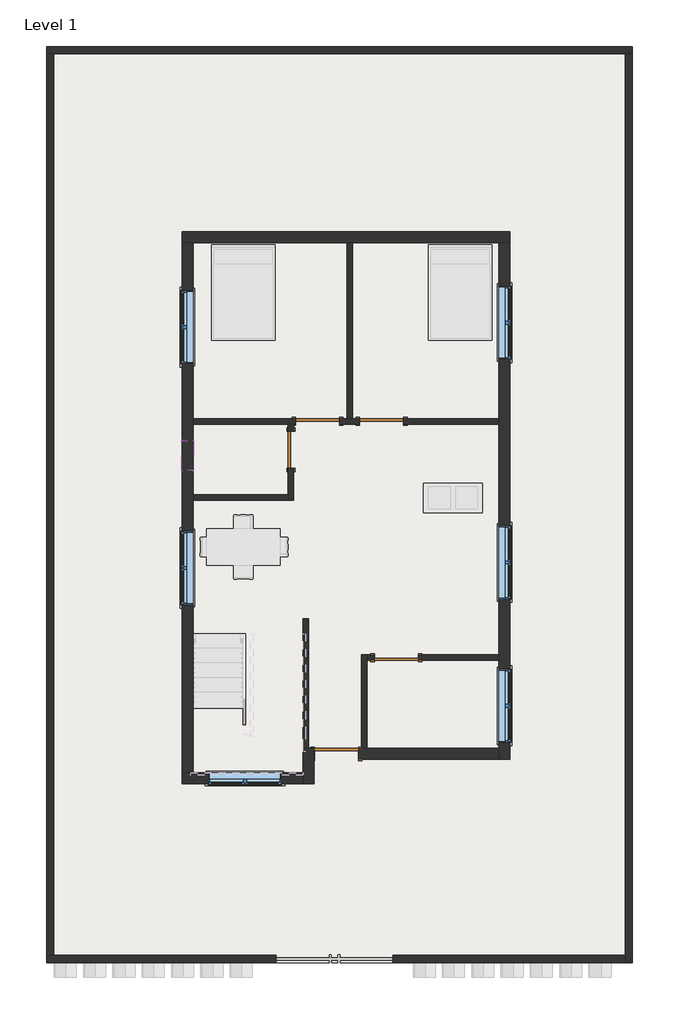
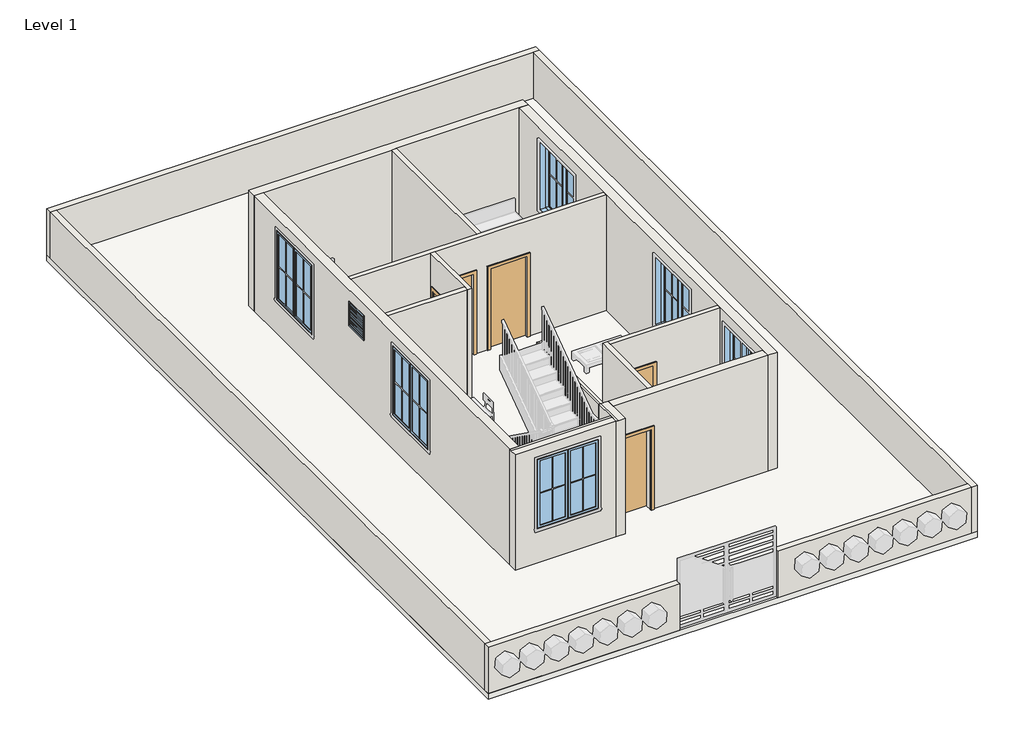
# One storey, part 1 of 3: 18 walls, 7 windows, 5 doors, 1 slab.
"""IFC4 building model written with IfcOpenShell, lengths in millimetres."""

from ifc_helpers import new_model, si_unit, frame, origin, origin_with_axes, place, context, project, spatial, polyline, outline, extrude, faceted_brep, transform, mapped, element, save
from components import door_214872d5, single_flush_door_3_e5f9f3c4, single_flush_door_3_305aa2a5, single_flush_door_3_0ca8825f, window_casement_double_win_5_f93960c7, window_f2d8fef0

model = new_model("IFC4")

# Units and contexts
model_context = context("Model", 3, world=origin())
ifc_project = project(units=[si_unit("LENGTHUNIT", "METRE", prefix="MILLI")], contexts=[model_context])

# Site, building, storey
site = spatial("IfcSite", under=ifc_project)
building = spatial("IfcBuilding", under=site)
storey = spatial("IfcBuildingStorey", under=building, Name="Level 1", Elevation=0.0)

# Doors
placement = place(None, origin())
door_shape = door_214872d5(model_context)
element("IfcDoor", 1, ObjectType="Single-Flush : DOOR 2'6\"", at=placement, inside=storey, context=model_context, shape_type="MappedRepresentation", body=[
    mapped(door_shape, transform((-2193.930864, 251.0919982, 0.0), x_axis=(0.0, 1.0, 0.0), y_axis=(-1.0, 0.0, 0.0), z_axis=(0.0, 0.0, 1.0))),
])
single_flush_door_3_shape = single_flush_door_3_e5f9f3c4(model_context)
element("IfcDoor", 2, ObjectType="Single-Flush : DOOR 3'", at=placement, inside=storey, context=model_context, shape_type="MappedRepresentation", body=[
    mapped(single_flush_door_3_shape, transform((-1641.3962678, 841.6419982, 0.0), x_axis=(1.0, 0.0, 0.0), y_axis=(0.0, 1.0, 0.0), z_axis=(0.0, 0.0, 1.0))),
])
element("IfcDoor", 3, ObjectType="Single-Flush : DOOR 3'", at=placement, inside=storey, context=model_context, shape_type="MappedRepresentation", body=[
    mapped(single_flush_door_3_shape, transform((-3.180864, -4073.2580018, 0.0), x_axis=(-1.0, 0.0, 0.0), y_axis=(0.0, -1.0, 0.0), z_axis=(0.0, 0.0, 1.0))),
])
single_flush_door_3_2_shape = single_flush_door_3_305aa2a5(model_context)
element("IfcDoor", 4, ObjectType="Single-Flush : DOOR 3'", at=placement, inside=storey, context=model_context, shape_type="MappedRepresentation", body=[
    mapped(single_flush_door_3_2_shape, transform((-307.980864, 841.6419982, 0.0), x_axis=(-1.0, 0.0, 0.0), y_axis=(0.0, -1.0, 0.0), z_axis=(0.0, 0.0, 1.0))),
])
single_flush_door_3_3_shape = single_flush_door_3_0ca8825f(model_context)
element("IfcDoor", 5, ObjectType="Single-Flush : DOOR 3'", at=placement, inside=storey, context=model_context, shape_type="MappedRepresentation", body=[
    mapped(single_flush_door_3_3_shape, transform((-1250.955864, -6073.5080018, 0.0), x_axis=(1.0, 0.0, 0.0), y_axis=(0.0, 1.0, 0.0), z_axis=(0.0, 0.0, 1.0))),
])

# Slab
element("IfcSlab", 6, ObjectType="FLOOR 6\"", at=placement, inside=storey, context=model_context, shape_type="SweptSolid", body=[
    extrude(outline(polyline([(4911.0485399, 8634.4627566), (4911.0485399, -10415.5372434), (-7280.9514601, -10415.5372434), (-7280.9514601, 8634.4627566), (4911.0485399, 8634.4627566)])), frame((0.0, 0.0, -152.4), z_axis=(0.0, 0.0, 1.0), x_axis=(1.0, 0.0, 0.0)), (0.0, 0.0, 1.0), 152.4),
])

# Walls
element("IfcWall", 7, ObjectType="CMD 6\"", at=placement, inside=storey, context=model_context, shape_type="Brep", body=[
    faceted_brep([(-7280.9514601, 8482.0627566, 0.0), (-7128.5514601, 8482.0627566, 0.0), (4758.6485399, 8482.0627566, 0.0), (4911.0485399, 8482.0627566, 0.0), (4911.0485399, 8482.0627566, 1219.2), (4758.6485399, 8482.0627566, 1219.2), (-7128.5514601, 8482.0627566, 1219.2), (-7280.9514601, 8482.0627566, 1219.2), (-7280.9514601, 8634.4627566, 0.0), (-7280.9514601, 8634.4627566, 1219.2), (4911.0485399, 8634.4627566, 1219.2), (4911.0485399, 8634.4627566, 0.0)], [[[0, 1, 2, 3, 4, 5, 6, 7]], [[8, 9, 10, 11]], [[3, 2, 1, 0, 8, 11]], [[7, 6, 5, 4, 10, 9]], [[4, 3, 11, 10]], [[0, 7, 9, 8]]]),
])
element("IfcWall", 8, ObjectType="CMD 6\"", at=placement, inside=storey, context=model_context, shape_type="Brep", body=[
    faceted_brep([(4758.6485399, 8482.0627566, 0.0), (4758.6485399, -10263.1372434, 0.0), (4758.6485399, -10415.5372434, 0.0), (4758.6485399, -10415.5372434, 1219.2), (4758.6485399, -10263.1372434, 1219.2), (4758.6485399, 8482.0627566, 1219.2), (4911.0485399, 8482.0627566, 0.0), (4911.0485399, 8482.0627566, 1219.2), (4911.0485399, -10415.5372434, 1219.2), (4911.0485399, -10415.5372434, 0.0)], [[[0, 1, 2, 3, 4, 5]], [[6, 7, 8, 9]], [[2, 1, 0, 6, 9]], [[5, 4, 3, 8, 7]], [[0, 5, 7, 6]], [[3, 2, 9, 8]]]),
])
element("IfcWall", 9, ObjectType="CMD 6\"", at=placement, inside=storey, context=model_context, shape_type="SweptSolid", body=[
    extrude(outline(polyline([(-67.3514601, -10263.1372434), (4758.6485399, -10263.1372434), (4758.6485399, -10415.5372434), (-67.3514601, -10415.5372434), (-67.3514601, -10263.1372434)])), origin_with_axes(), (0.0, 0.0, 1.0), 1219.2),
])
element("IfcWall", 10, ObjectType="CMD 6\"", at=placement, inside=storey, context=model_context, shape_type="SweptSolid", body=[
    extrude(outline(polyline([(-7128.5514601, 8482.0627566), (-7128.5514601, -10263.1372434), (-7280.9514601, -10263.1372434), (-7280.9514601, 8482.0627566), (-7128.5514601, 8482.0627566)])), origin_with_axes(), (0.0, 0.0, 1.0), 1219.2),
])
element("IfcWall", 11, ObjectType="CMD 6\"", at=placement, inside=storey, context=model_context, shape_type="Brep", body=[
    faceted_brep([(-2505.7514601, -10263.1372434, 0.0), (-7128.5514601, -10263.1372434, 0.0), (-7280.9514601, -10263.1372434, 0.0), (-7280.9514601, -10263.1372434, 1219.2), (-7128.5514601, -10263.1372434, 1219.2), (-2505.7514601, -10263.1372434, 1219.2), (-2505.7514601, -10415.5372434, 0.0), (-2505.7514601, -10415.5372434, 1219.2), (-7280.9514601, -10415.5372434, 1219.2), (-7280.9514601, -10415.5372434, 0.0)], [[[0, 1, 2, 3, 4, 5]], [[6, 7, 8, 9]], [[2, 1, 0, 6, 9]], [[5, 4, 3, 8, 7]], [[0, 5, 7, 6]], [[3, 2, 9, 8]]]),
])
element("IfcWall", 12, ObjectType="WALL 4.5\"", at=placement, inside=storey, context=model_context, shape_type="SweptSolid", body=[
    extrude(outline(polyline([(-1031.880864, 898.7919982), (-1031.880864, 4556.3919982), (-917.580864, 4556.3919982), (-917.580864, 898.7919982), (-1031.880864, 898.7919982)])), origin_with_axes(), (0.0, 0.0, 1.0), 3048.0),
])
element("IfcWall", 13, ObjectType="WALL 4.5\"", at=placement, inside=storey, context=model_context, shape_type="Brep", body=[
    faceted_brep([(-765.180864, 898.7919982, 2133.6), (-765.180864, 898.7919982, 0.0), (-917.580864, 898.7919982, 0.0), (-1031.880864, 898.7919982, 0.0), (-1184.1962678, 898.7919982, 0.0), (-1184.1962678, 898.7919982, 2133.6), (-2098.5962678, 898.7919982, 2133.6), (-2098.5962678, 898.7919982, 0.0), (-4232.280864, 898.7919982, 0.0), (-4232.280864, 898.7919982, 3048.0), (-1031.880864, 898.7919982, 3048.0), (-917.580864, 898.7919982, 3048.0), (2130.419136, 898.7919982, 3048.0), (2130.419136, 898.7919982, 0.0), (149.219136, 898.7919982, 0.0), (149.219136, 898.7919982, 2133.6), (-1184.1962678, 784.4919982, 0.0), (-765.180864, 784.4919982, 0.0), (-765.180864, 784.4919982, 2133.6), (149.219136, 784.4919982, 2133.6), (149.219136, 784.4919982, 0.0), (2130.419136, 784.4919982, 0.0), (2130.419136, 784.4919982, 3048.0), (-2136.780864, 784.4919982, 3048.0), (-2251.080864, 784.4919982, 3048.0), (-4232.280864, 784.4919982, 3048.0), (-4232.280864, 784.4919982, 0.0), (-2251.080864, 784.4919982, 0.0), (-2136.780864, 784.4919982, 0.0), (-2098.5962678, 784.4919982, 0.0), (-2098.5962678, 784.4919982, 2133.6), (-1184.1962678, 784.4919982, 2133.6)], [[[0, 1, 2, 3, 4, 5, 6, 7, 8, 9, 10, 11, 12, 13, 14, 15]], [[16, 17, 18, 19, 20, 21, 22, 23, 24, 25, 26, 27, 28, 29, 30, 31]], [[29, 28, 27, 26, 8, 7]], [[14, 13, 21, 20]], [[4, 3, 2, 1, 17, 16]], [[13, 12, 22, 21]], [[9, 8, 26, 25]], [[5, 4, 16, 31]], [[6, 5, 31, 30]], [[7, 6, 30, 29]], [[18, 17, 1, 0]], [[19, 18, 0, 15]], [[20, 19, 15, 14]], [[12, 11, 10, 9, 25, 24, 23, 22]]]),
])
element("IfcWall", 14, ObjectType="WALL 4.5\"", at=placement, inside=storey, context=model_context, shape_type="Brep", body=[
    faceted_brep([(-2251.080864, 784.4919982, 0.0), (-2251.080864, 632.0919982, 0.0), (-2251.080864, 632.0919982, 2133.6), (-2251.080864, -129.9080018, 2133.6), (-2251.080864, -129.9080018, 0.0), (-2251.080864, -688.7080018, 0.0), (-2251.080864, -803.0080018, 0.0), (-2251.080864, -803.0080018, 3048.0), (-2251.080864, -688.7080018, 3048.0), (-2251.080864, 784.4919982, 3048.0), (-2136.780864, 632.0919982, 2133.6), (-2136.780864, 632.0919982, 0.0), (-2136.780864, 784.4919982, 0.0), (-2136.780864, 784.4919982, 3048.0), (-2136.780864, -803.0080018, 3048.0), (-2136.780864, -803.0080018, 0.0), (-2136.780864, -129.9080018, 0.0), (-2136.780864, -129.9080018, 2133.6)], [[[0, 1, 2, 3, 4, 5, 6, 7, 8, 9]], [[10, 11, 12, 13, 14, 15, 16, 17]], [[16, 15, 6, 5, 4]], [[12, 11, 1, 0]], [[0, 9, 13, 12]], [[7, 6, 15, 14]], [[2, 1, 11, 10]], [[3, 2, 10, 17]], [[4, 3, 17, 16]], [[9, 8, 7, 14, 13]]]),
])
element("IfcWall", 15, ObjectType="WALL 4.5\"", at=placement, inside=storey, context=model_context, shape_type="SweptSolid", body=[
    extrude(outline(polyline([(-4232.280864, -688.7080018), (-2251.080864, -688.7080018), (-2251.080864, -803.0080018), (-4232.280864, -803.0080018), (-4232.280864, -688.7080018)])), origin_with_axes(), (0.0, 0.0, 1.0), 3048.0),
])
element("IfcWall", 16, ObjectType="WALL 4.5\"", at=placement, inside=storey, context=model_context, shape_type="Brep", body=[
    faceted_brep([(-1831.980864, -5959.2080018, 0.0), (-1831.980864, -3266.8080018, 0.0), (-1831.980864, -3266.8080018, 3048.0), (-1831.980864, -5959.2080018, 3048.0), (-1946.280864, -5959.2080018, 0.0), (-1946.280864, -5959.2080018, 3048.0), (-1946.280864, -3266.8080018, 3048.0), (-1946.280864, -3266.8080018, 0.0), (-1895.480864, -3266.8080018, 3048.0), (-1895.480864, -5959.2080018, 3048.0), (-1895.480864, -3571.6080018, 3048.0)], [[[0, 1, 2, 3]], [[4, 5, 6, 7]], [[1, 0, 4, 7]], [[2, 1, 7, 6, 8]], [[0, 3, 9, 5, 4]], [[3, 2, 8, 10, 9]], [[8, 6, 5, 9, 10]]]),
])
element("IfcWall", 17, ObjectType="WALL 4.5\"", at=placement, inside=storey, context=model_context, shape_type="Brep", body=[
    faceted_brep([(-612.780864, -5959.2080018, 0.0), (-612.780864, -4130.4080018, 0.0), (-612.780864, -4016.1080018, 0.0), (-612.780864, -4016.1080018, 3048.0), (-612.780864, -4130.4080018, 3048.0), (-612.780864, -5959.2080018, 3048.0), (-727.080864, -5959.2080018, 0.0), (-727.080864, -5959.2080018, 3048.0), (-727.080864, -4016.1080018, 3048.0), (-727.080864, -4016.1080018, 0.0)], [[[0, 1, 2, 3, 4, 5]], [[6, 7, 8, 9]], [[2, 1, 0, 6, 9]], [[0, 5, 7, 6]], [[3, 2, 9, 8]], [[5, 4, 3, 8, 7]]]),
])
element("IfcWall", 18, ObjectType="WALL 4.5\"", at=placement, inside=storey, context=model_context, shape_type="SweptSolid", body=[
    extrude(outline(polyline([(0.0, -612.780864), (0.0, -460.380864), (2133.6, -460.380864), (2133.6, 454.019136), (0.0, 454.019136), (0.0, 2130.419136), (3048.0, 2130.419136), (3048.0, -612.780864), (0.0, -612.780864)])), frame((0.0, -4130.4080018, 0.0), z_axis=(0.0, 1.0, 0.0), x_axis=(0.0, 0.0, 1.0)), (0.0, 0.0, 1.0), 114.3),
])
element("IfcWall", 19, ObjectType="WALL 9\"", at=placement, inside=storey, context=model_context, shape_type="Brep", body=[
    faceted_brep([(-4460.880864, 4556.3919982, 0.0), (-4232.280864, 4556.3919982, 0.0), (-1031.880864, 4556.3919982, 0.0), (-917.580864, 4556.3919982, 0.0), (2130.419136, 4556.3919982, 0.0), (2359.019136, 4556.3919982, 0.0), (2359.019136, 4556.3919982, 3048.0), (2130.419136, 4556.3919982, 3048.0), (-917.580864, 4556.3919982, 3048.0), (-1031.880864, 4556.3919982, 3048.0), (-4232.280864, 4556.3919982, 3048.0), (-4460.880864, 4556.3919982, 3048.0), (-4460.880864, 4784.9919982, 0.0), (-4460.880864, 4784.9919982, 3048.0), (2359.019136, 4784.9919982, 3048.0), (2359.019136, 4784.9919982, 0.0)], [[[0, 1, 2, 3, 4, 5, 6, 7, 8, 9, 10, 11]], [[12, 13, 14, 15]], [[5, 4, 3, 2, 1, 0, 12, 15]], [[6, 5, 15, 14]], [[0, 11, 13, 12]], [[11, 10, 9, 8, 7, 6, 14, 13]]]),
])
element("IfcWall", 20, ObjectType="WALL 9\"", at=placement, inside=storey, context=model_context, shape_type="Brep", body=[
    faceted_brep([(2130.419136, 4556.3919982, 0.0), (2130.419136, 898.7919982, 0.0), (2130.419136, 784.4919982, 0.0), (2130.419136, -4016.1080018, 0.0), (2130.419136, -4130.4080018, 0.0), (2130.419136, -5959.2080018, 0.0), (2130.419136, -6187.8080018, 0.0), (2130.419136, -6187.8080018, 3048.0), (2130.419136, -5959.2080018, 3048.0), (2130.419136, -4130.4080018, 3048.0), (2130.419136, -4016.1080018, 3048.0), (2130.419136, 784.4919982, 3048.0), (2130.419136, 898.7919982, 3048.0), (2130.419136, 4556.3919982, 3048.0), (2130.419136, -5835.3830018, 2743.2), (2130.419136, -5835.3830018, 914.4), (2130.419136, -4311.3830018, 914.4), (2130.419136, -4311.3830018, 2743.2), (2130.419136, -2854.0580018, 2743.2), (2130.419136, -2854.0580018, 914.4), (2130.419136, -1330.0580018, 914.4), (2130.419136, -1330.0580018, 2743.2), (2130.419136, 2130.6919982, 2743.2), (2130.419136, 2130.6919982, 914.4), (2130.419136, 3654.6919982, 914.4), (2130.419136, 3654.6919982, 2743.2), (2359.019136, 4556.3919982, 0.0), (2359.019136, 4556.3919982, 3048.0), (2359.019136, -6187.8080018, 3048.0), (2359.019136, -6187.8080018, 0.0), (2359.019136, -5835.3830018, 2743.2), (2359.019136, -4311.3830018, 2743.2), (2359.019136, -4311.3830018, 914.4), (2359.019136, -5835.3830018, 914.4), (2359.019136, -2854.0580018, 2743.2), (2359.019136, -1330.0580018, 2743.2), (2359.019136, -1330.0580018, 914.4), (2359.019136, -2854.0580018, 914.4), (2359.019136, 2130.6919982, 2743.2), (2359.019136, 3654.6919982, 2743.2), (2359.019136, 3654.6919982, 914.4), (2359.019136, 2130.6919982, 914.4)], [[[0, 1, 2, 3, 4, 5, 6, 7, 8, 9, 10, 11, 12, 13], [14, 15, 16, 17], [18, 19, 20, 21], [22, 23, 24, 25]], [[26, 27, 28, 29], [30, 31, 32, 33], [34, 35, 36, 37], [38, 39, 40, 41]], [[6, 5, 4, 3, 2, 1, 0, 26, 29]], [[0, 13, 27, 26]], [[7, 6, 29, 28]], [[15, 14, 30, 33]], [[16, 15, 33, 32]], [[17, 16, 32, 31]], [[14, 17, 31, 30]], [[19, 18, 34, 37]], [[20, 19, 37, 36]], [[21, 20, 36, 35]], [[18, 21, 35, 34]], [[23, 22, 38, 41]], [[24, 23, 41, 40]], [[25, 24, 40, 39]], [[22, 25, 39, 38]], [[13, 12, 11, 10, 9, 8, 7, 28, 27]]]),
])
element("IfcWall", 21, ObjectType="WALL 9\"", at=placement, inside=storey, context=model_context, shape_type="Brep", body=[
    faceted_brep([(2130.419136, -5959.2080018, 0.0), (-612.780864, -5959.2080018, 0.0), (-727.080864, -5959.2080018, 0.0), (-793.755864, -5959.2080018, 0.0), (-793.755864, -5959.2080018, 2133.6), (-1708.155864, -5959.2080018, 2133.6), (-1708.155864, -5959.2080018, 0.0), (-1717.680864, -5959.2080018, 0.0), (-1717.680864, -5959.2080018, 3048.0), (-727.080864, -5959.2080018, 3048.0), (-612.780864, -5959.2080018, 3048.0), (2130.419136, -5959.2080018, 3048.0), (-793.755864, -6187.8080018, 2133.6), (-793.755864, -6187.8080018, 0.0), (2130.419136, -6187.8080018, 0.0), (2130.419136, -6187.8080018, 3048.0), (-1717.680864, -6187.8080018, 3048.0), (-1717.680864, -6187.8080018, 0.0), (-1708.155864, -6187.8080018, 0.0), (-1708.155864, -6187.8080018, 2133.6)], [[[0, 1, 2, 3, 4, 5, 6, 7, 8, 9, 10, 11]], [[12, 13, 14, 15, 16, 17, 18, 19]], [[18, 17, 7, 6]], [[14, 13, 3, 2, 1, 0]], [[0, 11, 15, 14]], [[8, 7, 17, 16]], [[4, 3, 13, 12]], [[5, 4, 12, 19]], [[6, 5, 19, 18]], [[11, 10, 9, 8, 16, 15]]]),
])
element("IfcWall", 22, ObjectType="WALL 9\"", at=placement, inside=storey, context=model_context, shape_type="Brep", body=[
    faceted_brep([(-1946.280864, -5959.2080018, 0.0), (-1946.280864, -6467.2080018, 0.0), (-1946.280864, -6695.8080018, 0.0), (-1946.280864, -6695.8080018, 3048.0), (-1946.280864, -6467.2080018, 3048.0), (-1946.280864, -5959.2080018, 3048.0), (-1717.680864, -5959.2080018, 0.0), (-1717.680864, -5959.2080018, 3048.0), (-1717.680864, -6187.8080018, 3048.0), (-1717.680864, -6695.8080018, 3048.0), (-1717.680864, -6695.8080018, 0.0), (-1717.680864, -6187.8080018, 0.0), (-1831.980864, -5959.2080018, 0.0), (-1895.480864, -5959.2080018, 3048.0), (-1831.980864, -5959.2080018, 3048.0), (-1895.480864, -6695.8080018, 3048.0), (-1895.480864, -6518.0080018, 3048.0)], [[[0, 1, 2, 3, 4, 5]], [[6, 7, 8, 9, 10, 11]], [[2, 1, 0, 12, 6, 11, 10]], [[0, 5, 13, 14, 7, 6, 12]], [[3, 2, 10, 9, 15]], [[5, 4, 3, 15, 16, 13]], [[15, 9, 8, 7, 14, 13, 16]]]),
])
element("IfcWall", 23, ObjectType="WALL 9\"", at=placement, inside=storey, context=model_context, shape_type="Brep", body=[
    faceted_brep([(-1946.280864, -6467.2080018, 0.0), (-4232.280864, -6467.2080018, 0.0), (-4460.880864, -6467.2080018, 0.0), (-4460.880864, -6467.2080018, 3048.0), (-4232.280864, -6467.2080018, 3048.0), (-1946.280864, -6467.2080018, 3048.0), (-3914.780864, -6467.2080018, 2743.2), (-3914.780864, -6467.2080018, 914.4), (-2390.780864, -6467.2080018, 914.4), (-2390.780864, -6467.2080018, 2743.2), (-1946.280864, -6695.8080018, 0.0), (-1946.280864, -6695.8080018, 3048.0), (-4460.880864, -6695.8080018, 3048.0), (-4460.880864, -6695.8080018, 0.0), (-3914.780864, -6695.8080018, 2743.2), (-2390.780864, -6695.8080018, 2743.2), (-2390.780864, -6695.8080018, 914.4), (-3914.780864, -6695.8080018, 914.4), (-1946.280864, -6518.0080018, 3048.0), (-4460.880864, -6518.0080018, 3048.0), (-4232.280864, -6518.0080018, 3048.0)], [[[0, 1, 2, 3, 4, 5], [6, 7, 8, 9]], [[10, 11, 12, 13], [14, 15, 16, 17]], [[2, 1, 0, 10, 13]], [[0, 5, 18, 11, 10]], [[3, 2, 13, 12, 19]], [[7, 6, 14, 17]], [[8, 7, 17, 16]], [[9, 8, 16, 15]], [[6, 9, 15, 14]], [[5, 4, 3, 19, 20, 18]], [[19, 12, 11, 18, 20]]]),
])
element("IfcWall", 24, ObjectType="WALL 9\"", at=placement, inside=storey, context=model_context, shape_type="Brep", body=[
    faceted_brep([(-4232.280864, -6467.2080018, 0.0), (-4232.280864, -803.0080018, 0.0), (-4232.280864, -688.7080018, 0.0), (-4232.280864, 784.4919982, 0.0), (-4232.280864, 898.7919982, 0.0), (-4232.280864, 4556.3919982, 0.0), (-4232.280864, 4556.3919982, 3048.0), (-4232.280864, 898.7919982, 3048.0), (-4232.280864, 784.4919982, 3048.0), (-4232.280864, -688.7080018, 3048.0), (-4232.280864, -803.0080018, 3048.0), (-4232.280864, -3571.6080018, 3048.0), (-4232.280864, -6467.2080018, 3048.0), (-4232.280864, -1445.1400081, 2743.2), (-4232.280864, -1445.1400081, 914.4), (-4232.280864, -2969.1400081, 914.4), (-4232.280864, -2969.1400081, 2743.2), (-4232.280864, 3562.6287133, 2743.2), (-4232.280864, 3562.6287133, 914.4), (-4232.280864, 2038.6287133, 914.4), (-4232.280864, 2038.6287133, 2743.2), (-4232.280864, -174.3580018, 2743.2), (-4232.280864, 435.2419982, 2743.2), (-4232.280864, 435.2419982, 2133.6), (-4232.280864, -174.3580018, 2133.6), (-4460.880864, -6467.2080018, 0.0), (-4460.880864, -6467.2080018, 3048.0), (-4460.880864, 4556.3919982, 3048.0), (-4460.880864, 4556.3919982, 0.0), (-4460.880864, -1445.1400081, 2743.2), (-4460.880864, -2969.1400081, 2743.2), (-4460.880864, -2969.1400081, 914.4), (-4460.880864, -1445.1400081, 914.4), (-4460.880864, 3562.6287133, 2743.2), (-4460.880864, 2038.6287133, 2743.2), (-4460.880864, 2038.6287133, 914.4), (-4460.880864, 3562.6287133, 914.4), (-4460.880864, -174.3580018, 2743.2), (-4460.880864, -174.3580018, 2133.6), (-4460.880864, 435.2419982, 2133.6), (-4460.880864, 435.2419982, 2743.2)], [[[0, 1, 2, 3, 4, 5, 6, 7, 8, 9, 10, 11, 12], [13, 14, 15, 16], [17, 18, 19, 20], [21, 22, 23, 24]], [[25, 26, 27, 28], [29, 30, 31, 32], [33, 34, 35, 36], [37, 38, 39, 40]], [[5, 4, 3, 2, 1, 0, 25, 28]], [[6, 5, 28, 27]], [[0, 12, 26, 25]], [[14, 13, 29, 32]], [[15, 14, 32, 31]], [[16, 15, 31, 30]], [[13, 16, 30, 29]], [[18, 17, 33, 36]], [[19, 18, 36, 35]], [[20, 19, 35, 34]], [[17, 20, 34, 33]], [[38, 37, 21, 24]], [[39, 38, 24, 23]], [[40, 39, 23, 22]], [[37, 40, 22, 21]], [[12, 11, 10, 9, 8, 7, 6, 27, 26]]]),
])

# Windows
window_casement_double_win_5_shape = window_casement_double_win_5_f93960c7(model_context)
element("IfcWindow", 25, ObjectType="Window-Casement-Double : WIN 5'", at=placement, inside=storey, context=model_context, shape_type="MappedRepresentation", body=[
    mapped(window_casement_double_win_5_shape, transform((-3152.780864, -6581.5080018, 0.0), x_axis=(-1.0, 0.0, 0.0), y_axis=(0.0, -1.0, 0.0), z_axis=(0.0, 0.0, 1.0))),
])
element("IfcWindow", 26, ObjectType="Window-Casement-Double : WIN 5'", at=placement, inside=storey, context=model_context, shape_type="MappedRepresentation", body=[
    mapped(window_casement_double_win_5_shape, transform((2244.719136, -5073.3830018, 0.0), x_axis=(0.0, -1.0, 0.0), y_axis=(1.0, 0.0, 0.0), z_axis=(0.0, 0.0, 1.0))),
])
element("IfcWindow", 27, ObjectType="Window-Casement-Double : WIN 5'", at=placement, inside=storey, context=model_context, shape_type="MappedRepresentation", body=[
    mapped(window_casement_double_win_5_shape, transform((2244.719136, -2092.0580018, 0.0), x_axis=(0.0, -1.0, 0.0), y_axis=(1.0, 0.0, 0.0), z_axis=(0.0, 0.0, 1.0))),
])
element("IfcWindow", 28, ObjectType="Window-Casement-Double : WIN 5'", at=placement, inside=storey, context=model_context, shape_type="MappedRepresentation", body=[
    mapped(window_casement_double_win_5_shape, transform((-4346.580864, -2207.1400081, 0.0), x_axis=(0.0, 1.0, 0.0), y_axis=(-1.0, 0.0, 0.0), z_axis=(0.0, 0.0, 1.0))),
])
element("IfcWindow", 29, ObjectType="Window-Casement-Double : WIN 5'", at=placement, inside=storey, context=model_context, shape_type="MappedRepresentation", body=[
    mapped(window_casement_double_win_5_shape, transform((2244.719136, 2892.6919982, 0.0), x_axis=(0.0, -1.0, 0.0), y_axis=(1.0, 0.0, 0.0), z_axis=(0.0, 0.0, 1.0))),
])
element("IfcWindow", 30, ObjectType="Window-Casement-Double : WIN 5'", at=placement, inside=storey, context=model_context, shape_type="MappedRepresentation", body=[
    mapped(window_casement_double_win_5_shape, transform((-4346.580864, 2800.6287133, 0.0), x_axis=(0.0, 1.0, 0.0), y_axis=(-1.0, 0.0, 0.0), z_axis=(0.0, 0.0, 1.0))),
])
window_shape = window_f2d8fef0(model_context)
element("IfcWindow", 31, ObjectType="Window-Louvers : 24\" x 24\"", at=placement, inside=storey, context=model_context, shape_type="MappedRepresentation", body=[
    mapped(window_shape, transform((-4352.930864, 130.4419982, 1219.2), x_axis=(0.0, 1.0, 0.0), y_axis=(-1.0, 0.0, 0.0), z_axis=(0.0, 0.0, 1.0))),
])

save(model, "model.ifc")

# Revit data of these elements
# Type "Single-Flush : DOOR 2'6\""
#   Type Mark = "9"
#   Construction Type Id = "MDOOR"
#   Assembly Code = "C1020"
#   Analytic Construction = "Metal"
#   Thickness = 0' - 2"
#   Heat Transfer Coefficient (U) = 0.651978 BTU/(h·ft²·°F)
#   Height = 7' - 0"
#   Trim Projection Ext = 0' - 1"
#   Trim Projection Int = 0' - 1"
#   Trim Width = 0' - 3"
#   Width = 2' - 6"
#   Define Thermal Properties by = 1
#   Door Material = Door - Panel
#   Frame Material = Door - Frame
#   Visual Light Transmittance = 0
#   Solar Heat Gain Coefficient = 0
#   Function = (empty or 0)
#   Wall Closure = (empty or 0)
# Type "Single-Flush : DOOR 3'"
#   Type Mark = "8"
#   Construction Type Id = "MDOOR"
#   Assembly Code = "C1020"
#   Analytic Construction = "Metal"
#   Thickness = 0' - 2"
#   Heat Transfer Coefficient (U) = 0.651978 BTU/(h·ft²·°F)
#   Height = 7' - 0"
#   Trim Projection Ext = 0' - 1"
#   Trim Projection Int = 0' - 1"
#   Trim Width = 0' - 3"
#   Width = 3' - 0"
#   Define Thermal Properties by = 1
#   Door Material = Door - Panel
#   Frame Material = Door - Frame
#   Visual Light Transmittance = 0
#   Solar Heat Gain Coefficient = 0
#   Function = (empty or 0)
#   Wall Closure = (empty or 0)
# Type "FLOOR 6\""
#   Assembly Code = "B1010"
#   Function = 0
#   Layers, outside or top first: 0' - 6" no material (function 1)
# Type "CMD 6\""
#   Assembly Code = "B2010"
#   Layers, outside or top first: 0' - 6" no material (function 1)
# Type "WALL 4.5\""
#   Assembly Code = "B2010"
#   Layers, outside or top first: 0' - 4 1/2" no material (function 1)
# Type "WALL 9\""
#   Assembly Code = "B2010"
#   Layers, outside or top first: 0' - 9" no material (function 1)
# Type "Window-Casement-Double : WIN 5'"
#   Type Mark = "18"
#   Fire Rating = "0.5h"
#   Assembly Code = "B2020100"
#   Analytic Construction = "Double glazing - domestic"
#   Frame Extension [instance default] = 0' - 0 1/4"
#   Window Inset [instance default] = 0' - 0"
#   Wall Thickness [instance default] = 0' - 6"
#   Interior Wall Closure [instance default] = 0' - 2 1/4"
#   Half Width = 2' - 6"
#   Visual Light Transmittance = 0.81
#   Thermal Resistance (R) = 1.8146 (h·ft²·°F)/BTU
#   Solar Heat Gain Coefficient = 0.76
#   Rough Width = 5' - 0 1/2"
#   Rough Height = 6' - 0 1/2"
#   Height = 6' - 0"
#   Heat Transfer Coefficient (U) = 0.5511 BTU/(h·ft²·°F)
#   Exterior Wall Closure [instance default] = 0' - 1 1/4"
#   Extension Jamb [instance default] = 0' - 2 1/4"
#   Default Sill Height = 3' - 0"
#   Width = 5' - 0"
#   Muntin Visibility = yes
#   Interior Trim Visibility [instance default] = yes
#   Exterior Trim Visibility [instance default] = yes
#   Extension Jamb Visibility [instance default] = yes
#   Interior Trim Material = Wood - Stained
#   Muntin Pattern = Muntin Pattern_2x2 : Muntin Pattern_2x2
#   Interior Trim = Trim-Window-Interior-Flat : Picture Frame
#   Interior Frame Material = Wood - Stained
#   Glass Panel Material = Glass
#   Exterior Trim Material = Clad - White
#   Exterior Trim = Trim-Window-Exterior-Flat : with Sill
#   Exterior Frame Material = Clad - White
#   Wall Closure = (empty or 0)
# Type "Window-Louvers : 24\" x 24\""
#   Type Mark = "19"
#   Construction Type Id = "GSP4R"
#   Assembly Code = "B20"
#   Analytic Construction = "1/8 in Pilkington single glazing"
#   Visual Light Transmittance = 0.9
#   Thermal Resistance (R) = 1.53941 (h·ft²·°F)/BTU
#   Solar Heat Gain Coefficient = 0.78
#   Max Height = 1' - 11.74264"
#   Height = 2' - 0"
#   Heat Transfer Coefficient (U) = 0.6496 BTU/(h·ft²·°F)
#   Blade Width [instance default] = 1' - 10 1/2"
#   Blade Vertical Thickness = 0' - 0.35355"
#   Blade Thickness = 0' - 0 1/4"
#   Blade Spacing = 0' - 1 1/2"
#   Blade Height = 0' - 1.85355"
#   Blade Depth = 0' - 3"
#   Blade Angle = 45.00°
#   Default Sill Height = 3' - 0"
#   Trim Projection_Exterior = 0' - 0 1/2"
#   Trim Projection_Interior = 0' - 0 1/2"
#   Trim Width_Exterior = 0' - 1 1/2"
#   Trim Width_Interior = 0' - 1 1/2"
#   Width = 2' - 0"
#   Max Blade Count = 12
#   Define Thermal Properties by = 1
#   Blade Count = 12
#   Frame Material = Birch
#   Louver Material = Birch
#   Trim Exterior Material = Birch
#   Trim Interior Material = Birch
#   Wall Closure = (empty or 0)
# Element 1 (IfcDoor, "Single-Flush : DOOR 2'6\"")
#   Phase Created = New Construction
#   Materials on its faces: "Door - Frame", "Door - Panel"
# Elements 2, 3, 4, 5 (IfcDoor, "Single-Flush : DOOR 3'")
#   Phase Created = New Construction
#   Materials on its faces: "Door - Frame", "Door - Panel"
# Element 6 (IfcSlab, "FLOOR 6\"")
#   Height Offset From Level = 0' - 0"
#   Phase Created = New Construction
#   Materials on its faces: "Copper", "Default Floor", "Wood - Stained"
# Elements 7, 8, 9 (IfcWall, "CMD 6\"")
#   Top Offset = 0' - 0"
#   Base Offset = 0' - 0"
#   Unconnected Height = 4' - 0"
#   wall height = 4' - 0"
#   Phase Created = New Construction
#   Base Constraint = Level 1
#   Materials on its faces: "Clad - White", "Default Wall", "Copper"
# Element 10 (IfcWall, "CMD 6\"")
#   Top Offset = 0' - 0"
#   Base Offset = 0' - 0"
#   Unconnected Height = 4' - 0"
#   wall height = 4' - 0"
#   Phase Created = New Construction
#   Base Constraint = Level 1
#   Materials on its faces: "Default Wall", "Clad - White", "Copper"
# Element 11 (IfcWall, "CMD 6\"")
#   Top Offset = 0' - 0"
#   Base Offset = 0' - 0"
#   Unconnected Height = 4' - 0"
#   wall height = 4' - 0"
#   Phase Created = New Construction
#   Base Constraint = Level 1
#   Materials on its faces: "Clad - White", "Copper", "Default Wall"
# Elements 12, 13, 14, 15, 17, 18 (IfcWall, "WALL 4.5\"")
#   Top Offset = 0' - 0"
#   Base Offset = 0' - 0"
#   Unconnected Height = 10' - 0"
#   wall height = 10' - 0"
#   Phase Created = New Construction
#   Base Constraint = Level 1
#   Materials on its faces: "Default Wall"
# Element 16 (IfcWall, "WALL 4.5\"")
#   Top Offset = 0' - 0"
#   Base Offset = 0' - 0"
#   Unconnected Height = 10' - 0"
#   wall height = 10' - 0"
#   Phase Created = New Construction
#   Base Constraint = Level 1
#   Materials on its faces: "Default Wall", "Copper"
# Elements 19, 20, 21 (IfcWall, "WALL 9\"")
#   Top Offset = 0' - 0"
#   Base Offset = 0' - 0"
#   Unconnected Height = 10' - 0"
#   wall height = 10' - 0"
#   Phase Created = New Construction
#   Base Constraint = Level 1
#   Materials on its faces: "Default Wall"
# Elements 22, 23, 24 (IfcWall, "WALL 9\"")
#   Top Offset = 0' - 0"
#   Base Offset = 0' - 0"
#   Unconnected Height = 10' - 0"
#   wall height = 10' - 0"
#   Phase Created = New Construction
#   Base Constraint = Level 1
#   Materials on its faces: "Default Wall", "Copper"
# Element 25 (IfcWindow, "Window-Casement-Double : WIN 5'")
#   Mark = "1"
#   Window Inset = 0' - 0"
#   Interior Wall Closure = 0' - 2 1/4"
#   Frame Extension = 0' - 0 1/4"
#   Exterior Wall Closure = 0' - 1 1/4"
#   Interior Trim Visibility = yes
#   Exterior Trim Visibility = yes
#   Phase Created = New Construction
#   Materials on its faces: "Wood - Stained", "Glass", "Clad - White"
# Element 26 (IfcWindow, "Window-Casement-Double : WIN 5'")
#   Mark = "2"
#   Window Inset = 0' - 0"
#   Interior Wall Closure = 0' - 2 1/4"
#   Frame Extension = 0' - 0 1/4"
#   Exterior Wall Closure = 0' - 1 1/4"
#   Interior Trim Visibility = yes
#   Exterior Trim Visibility = yes
#   Phase Created = New Construction
#   Materials on its faces: "Wood - Stained", "Glass", "Clad - White"
# Element 27 (IfcWindow, "Window-Casement-Double : WIN 5'")
#   Mark = "3"
#   Window Inset = 0' - 0"
#   Interior Wall Closure = 0' - 2 1/4"
#   Frame Extension = 0' - 0 1/4"
#   Exterior Wall Closure = 0' - 1 1/4"
#   Interior Trim Visibility = yes
#   Exterior Trim Visibility = yes
#   Phase Created = New Construction
#   Materials on its faces: "Wood - Stained", "Glass", "Clad - White"
# Element 28 (IfcWindow, "Window-Casement-Double : WIN 5'")
#   Mark = "4"
#   Window Inset = 0' - 0"
#   Interior Wall Closure = 0' - 2 1/4"
#   Frame Extension = 0' - 0 1/4"
#   Exterior Wall Closure = 0' - 1 1/4"
#   Interior Trim Visibility = yes
#   Exterior Trim Visibility = yes
#   Phase Created = New Construction
#   Materials on its faces: "Wood - Stained", "Glass", "Clad - White"
# Element 29 (IfcWindow, "Window-Casement-Double : WIN 5'")
#   Mark = "5"
#   Window Inset = 0' - 0"
#   Interior Wall Closure = 0' - 2 1/4"
#   Frame Extension = 0' - 0 1/4"
#   Exterior Wall Closure = 0' - 1 1/4"
#   Interior Trim Visibility = yes
#   Exterior Trim Visibility = yes
#   Phase Created = New Construction
#   Materials on its faces: "Wood - Stained", "Glass", "Clad - White"
# Element 30 (IfcWindow, "Window-Casement-Double : WIN 5'")
#   Mark = "6"
#   Window Inset = 0' - 0"
#   Interior Wall Closure = 0' - 2 1/4"
#   Frame Extension = 0' - 0 1/4"
#   Exterior Wall Closure = 0' - 1 1/4"
#   Interior Trim Visibility = yes
#   Exterior Trim Visibility = yes
#   Phase Created = New Construction
#   Materials on its faces: "Wood - Stained", "Glass", "Clad - White"
# Element 31 (IfcWindow, "Window-Louvers : 24\" x 24\"")
#   Mark = "7"
#   Blade Width = 1' - 10 1/2"
#   Phase Created = New Construction
#   Materials on its faces: "Birch"
# Materials
#   "Door - Panel": class "Wood", colour RGB 210 159 95, transparency 0, Cost = 0
#   "Door - Frame": colour RGB 118 70 51, transparency 0, Cost = 0
#   "Wood - Stained": class "Wood", colour RGB 224 178 126, transparency 0, Cost = 0
#   "Glass": class "Glass", colour RGB 0 128 192, transparency 0.75, Description = "Soda Lime Glass", Cost = 0
#   "Clad - White": class "Wood", colour RGB 242 242 238, transparency 0, Cost = 0
#   "Birch": class "Wood", colour RGB 224 178 126, transparency 0, Description = "Betula Alleghaniensis", Cost = 0
#   "Copper": class "Metal", colour RGB 0 0 0, transparency 0, Description = "Copper, matte finish", Cost = 0
#   "Default Floor": colour RGB 128 128 128, transparency 0, Cost = 0
#   "Default Wall": colour RGB 128 128 128, transparency 0, Cost = 0
